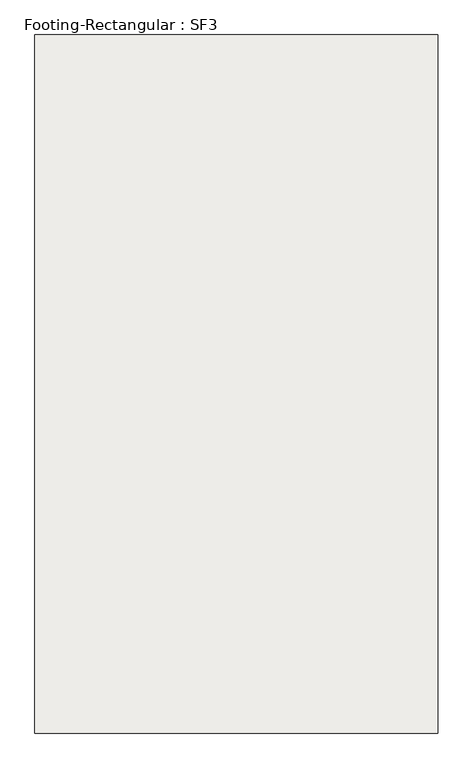
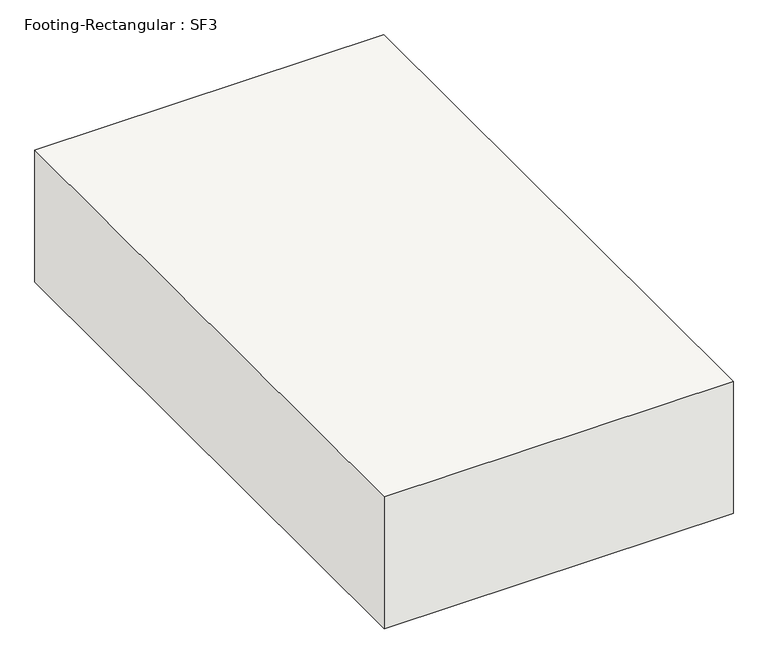
"""IFC4 building model written with IfcOpenShell, lengths in millimetres: slab geometry, Footing-Rectangular : SF3."""

from ifc_helpers import new_model, si_unit, frame, origin, place, context, project, spatial, polyline, outline, extrude, source, transform, mapped, element, save


def footing_rectangular_sf3_4ecd2a9c(model_context):
    return source(origin(), model_context, "Body", "SweptSolid", [
        extrude(outline(polyline([(571.5, 990.6), (571.5, -990.6), (-571.5, -990.6), (-571.5, 990.6), (571.5, 990.6)])), frame((0.0, 0.0, -457.2), z_axis=(0.0, 0.0, 1.0), x_axis=(1.0, 0.0, 0.0)), (0.0, 0.0, 1.0), 457.2),
    ])


if __name__ == "__main__":
    model = new_model("IFC4")
    model_context = context("Model", 3, world=origin())
    ifc_project = project(units=[si_unit("LENGTHUNIT", "METRE", prefix="MILLI")], contexts=[model_context])
    site = spatial("IfcSite", under=ifc_project)
    building = spatial("IfcBuilding", under=site)
    placement = place(None, origin())
    footing_rectangular_sf3_shape = footing_rectangular_sf3_4ecd2a9c(model_context)
    element("IfcSlab", 1, ObjectType="Footing-Rectangular : SF3", at=placement, inside=building, context=model_context, shape_type="MappedRepresentation", body=[
        mapped(footing_rectangular_sf3_shape, transform((0.0, 0.0, 0.0), x_axis=(1.0, 0.0, 0.0), y_axis=(0.0, 1.0, 0.0), z_axis=(0.0, 0.0, 1.0))),
    ])
    save(model, "model.ifc")

# Revit data of these elements
# Type "Footing-Rectangular : SF3"
#   Width = 1143 mm
#   Length = 1981.2 mm
#   Foundation Thickness = 457.2 mm
#   Structural Material [instance default] = Concrete - Cast-in-Place Concrete
#   Assembly Code = ""
# Element 1 (IfcSlab, "Footing-Rectangular : SF3")
#   Materials on its faces: "Concrete - Cast-in-Place Concrete"
# Materials
#   "Concrete - Cast-in-Place Concrete": class "Concrete", colour RGB 192 192 192, transparency 0, Cost = 0
